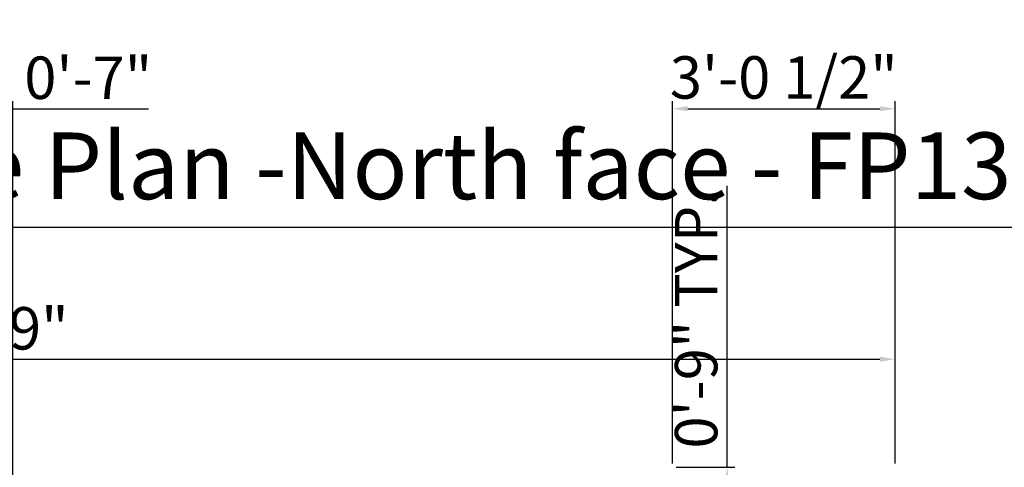
# Model space of a CAD drawing. Units: inches. Extents: x 1484 to 2008, y 1843 to 2590.
# Tile 19 of 21: x 1756 to 1918, y 2217 to 2291. Entities that reach past the tile are written whole.
import ezdxf

# ---------------------------------------------------------------- set-up
doc = ezdxf.new("R2010")
doc.units = ezdxf.units.IN
doc.layers.add('A-ANNO-DIMS', color=2, linetype='Continuous', lineweight=18)
doc.layers.add('A-ANNO-TEXT', color=7, linetype='Continuous', lineweight=25)
doc.styles.get("Standard").update_dxf_attribs({"font": 'arial.ttf'})
doc.dimstyles.new('ISO-25', dxfattribs={"dimtxt": 7, "dimasz": 2.5, "dimexe": 1.25, "dimexo": 0.625, "dimtad": 1, "dimdec": 0, "dimlunit": 3, "dimtxsty": 'Standard', "dimcen": 2.5, "dimadec": 0, "dimazin": 0, "dimtfac": 1, "dimtdec": 0, "dimtmove": 0, "dimatfit": 3, "dimfxl": 1, "dimarcsym": 0})

# ---------------------------------------------------------------- blocks, each defined once
blk = doc.blocks.new('*D2')
at = {"layer": 'A-ANNO-DIMS', "color": 0, "lineweight": -2, "transparency": 16777216}
for p, q in [((1602.92, 2217.93), (1602.92, 2236.39)), ((1899.92, 2217.93), (1899.92, 2236.39)), ((1605.42, 2235.14), (1897.42, 2235.14))]:
    blk.add_line(p, q, dxfattribs=at)
at = {"layer": 'A-ANNO-DIMS', "color": 0, "transparency": 16777216}
for points in [[(1605.42, 2235.55), (1605.42, 2234.72), (1602.92, 2235.14)], [(1897.42, 2235.55), (1897.42, 2234.72), (1899.92, 2235.14)]]:
    blk.add_solid(points, dxfattribs=at)
at = {"layer": 'Defpoints', "color": 0, "transparency": 16777216}
for p in [(1899.92, 2235.14), (1602.92, 2217.3), (1899.92, 2217.3)]:
    blk.add_point(p, dxfattribs=at)
at = {"layer": 'A-ANNO-DIMS', "color": 0, "transparency": 16777216, "insert": (1750.41, 2239.33), "char_height": 7, "attachment_point": 5}
blk.add_mtext('24\'-9"', dxfattribs=at)
blk = doc.blocks.new('*D13')
at = {"layer": 'A-ANNO-DIMS', "color": 0, "lineweight": -2, "transparency": 16777216}
for p, q in [((1803.22, 2207.68), (1803.22, 2198.05)), ((1863.22, 2207.68), (1863.22, 2198.05)), ((1805.72, 2199.3), (1860.72, 2199.3)), ((1863.22, 2199.3), (2008.2, 2199.3))]:
    blk.add_line(p, q, dxfattribs=at)
at = {"layer": 'A-ANNO-DIMS', "color": 0, "transparency": 16777216}
for points in [[(1805.72, 2199.72), (1805.72, 2198.89), (1803.22, 2199.3)], [(1860.72, 2199.72), (1860.72, 2198.89), (1863.22, 2199.3)]]:
    blk.add_solid(points, dxfattribs=at)
at = {"layer": 'Defpoints', "color": 0, "transparency": 16777216}
for p in [(1803.22, 2208.3), (1863.22, 2208.3), (1863.22, 2199.3)]:
    blk.add_point(p, dxfattribs=at)
at = {"layer": 'A-ANNO-DIMS', "color": 0, "transparency": 16777216, "insert": (1936.96, 2203.55), "char_height": 7, "attachment_point": 5}
blk.add_mtext('BEDROOM WINDOW 5\'-0" TYP.', dxfattribs=at)
blk = doc.blocks.new('*D14')
at = {"layer": 'A-ANNO-DIMS', "color": 0, "lineweight": -2, "transparency": 16777216}
for p, q in [((1872.22, 2217.3), (1872.22, 2263.72)), ((1863.84, 2217.3), (1873.47, 2217.3)), ((1872.22, 2210.8), (1872.22, 2214.8)), ((1863.84, 2208.3), (1873.47, 2208.3))]:
    blk.add_line(p, q, dxfattribs=at)
at = {"layer": 'A-ANNO-DIMS', "color": 0, "transparency": 16777216}
for points in [[(1871.8, 2214.8), (1872.64, 2214.8), (1872.22, 2217.3)], [(1871.8, 2210.8), (1872.64, 2210.8), (1872.22, 2208.3)]]:
    blk.add_solid(points, dxfattribs=at)
at = {"layer": 'Defpoints', "color": 0, "transparency": 16777216}
for p in [(1863.22, 2217.3), (1872.22, 2217.3), (1863.22, 2208.3)]:
    blk.add_point(p, dxfattribs=at)
at = {"layer": 'A-ANNO-DIMS', "color": 0, "transparency": 16777216, "insert": (1868.02, 2241.76), "char_height": 7, "attachment_point": 5, "rotation": 90}
blk.add_mtext('0\'-9" TYP.', dxfattribs=at)
blk = doc.blocks.new('*D28')
at = {"layer": 'A-ANNO-DIMS', "color": 0, "lineweight": -2, "transparency": 16777216}
for p, q in [((1863.22, 2217.93), (1863.22, 2277.72)), ((1899.92, 2217.93), (1899.92, 2277.72)), ((1865.72, 2276.47), (1897.42, 2276.47))]:
    blk.add_line(p, q, dxfattribs=at)
at = {"layer": 'A-ANNO-DIMS', "color": 0, "transparency": 16777216}
for points in [[(1865.72, 2276.89), (1865.72, 2276.06), (1863.22, 2276.47)], [(1897.42, 2276.89), (1897.42, 2276.06), (1899.92, 2276.47)]]:
    blk.add_solid(points, dxfattribs=at)
at = {"layer": 'Defpoints', "color": 0, "transparency": 16777216}
for p in [(1899.92, 2276.47), (1863.22, 2217.3), (1899.92, 2217.3)]:
    blk.add_point(p, dxfattribs=at)
at = {"layer": 'A-ANNO-DIMS', "color": 0, "transparency": 16777216, "insert": (1881.57, 2280.72), "char_height": 7, "attachment_point": 5}
blk.add_mtext('3\'-0 1/2"', dxfattribs=at)
blk = doc.blocks.new('*D38')
at = {"layer": 'A-ANNO-DIMS', "color": 0, "lineweight": -2, "transparency": 16777216}
for p, q in [((1747.43, 2141.93), (1747.43, 2277.72)), ((1754.42, 2141.93), (1754.42, 2277.72)), ((1749.93, 2276.47), (1751.92, 2276.47)), ((1754.42, 2276.47), (1776.78, 2276.47))]:
    blk.add_line(p, q, dxfattribs=at)
at = {"layer": 'A-ANNO-DIMS', "color": 0, "transparency": 16777216}
for points in [[(1749.93, 2276.89), (1749.93, 2276.06), (1747.43, 2276.47)], [(1751.92, 2276.89), (1751.92, 2276.06), (1754.42, 2276.47)]]:
    blk.add_solid(points, dxfattribs=at)
at = {"layer": 'Defpoints', "color": 0, "transparency": 16777216}
for p in [(1754.42, 2276.47), (1747.43, 2141.3), (1754.42, 2141.3)]:
    blk.add_point(p, dxfattribs=at)
at = {"layer": 'A-ANNO-DIMS', "color": 0, "transparency": 16777216, "insert": (1766.85, 2280.67), "char_height": 7, "attachment_point": 5}
blk.add_mtext('0\'-7"', dxfattribs=at)

msp = doc.modelspace()

# ---------------------------------------------------------------- linework, layer by layer
at = {"layer": 'A-ANNO-TEXT'}
msp.add_line((1588.86, 2256.92), (1942.3, 2256.92), dxfattribs=at)

# ---------------------------------------------------------------- texts
at = {"layer": 'A-ANNO-TEXT', "insert": (1591.11, 2272.55), "char_height": 11, "attachment_point": 1}
msp.add_mtext_dynamic_manual_height_columns('25X25 [625 sq ft ] House Plan -North face - FP1321', width=378.3718, gutter_width=12.5, heights=[0], dxfattribs=at)

# ---------------------------------------------------------------- dimensions: what is measured, and where the dimension line sits
at = {"layer": 'A-ANNO-DIMS'}
for base, p1, p2, picture, middle in [((1899.92, 2276.47), (1863.22, 2217.3), (1899.92, 2217.3), '*D28', (1881.57, 2280.72)), ((1754.42, 2276.47), (1747.43, 2141.3), (1754.42, 2141.3), '*D38', (1766.85, 2280.67))]:
    dim = msp.add_linear_dim(base=base, p1=p1, p2=p2, dimstyle='ISO-25', override={"dimdec": 1, "dimlfac": 1, "dimrnd": 0, "dimzin": 1, "dimdsep": 46, "dimlunit": 4, "dimfrac": 2}, dxfattribs=at)
    dim.commit()
    dim.dimension.update_dxf_attribs({"geometry": picture, "text_midpoint": middle})
dim = msp.add_linear_dim(base=(1872.22, 2217.3), p1=(1863.22, 2208.3), p2=(1863.22, 2217.3), angle=90, text='<> TYP.', dimstyle='ISO-25', override={"dimdec": 1, "dimlfac": 1, "dimrnd": 0, "dimzin": 1, "dimdsep": 46, "dimlunit": 4, "dimfrac": 2}, dxfattribs=at)
dim.commit()
dim.dimension.update_dxf_attribs({"geometry": '*D14', "text_midpoint": (1868.02, 2241.76)})
dim = msp.add_linear_dim(base=(1899.92, 2235.14), p1=(1602.92, 2217.3), p2=(1899.92, 2217.3), dimstyle='ISO-25', override={"dimclrd": 0, "dimclre": 0, "dimclrt": 0}, dxfattribs=at)
dim.commit()
dim.dimension.update_dxf_attribs({"geometry": '*D2', "text_midpoint": (1750.41, 2235.14), "dimtype": 160})
dim = msp.add_linear_dim(base=(1863.22, 2199.3), p1=(1803.22, 2208.3), p2=(1863.22, 2208.3), text='BEDROOM WINDOW <> TYP.', dimstyle='ISO-25', override={"dimdec": 1, "dimlfac": 1, "dimrnd": 0, "dimzin": 1, "dimdsep": 46, "dimlunit": 4, "dimfrac": 2}, dxfattribs=at)
dim.commit()
dim.dimension.update_dxf_attribs({"geometry": '*D13', "text_midpoint": (1936.96, 2203.55)})

doc.saveas('drawing.dxf')
